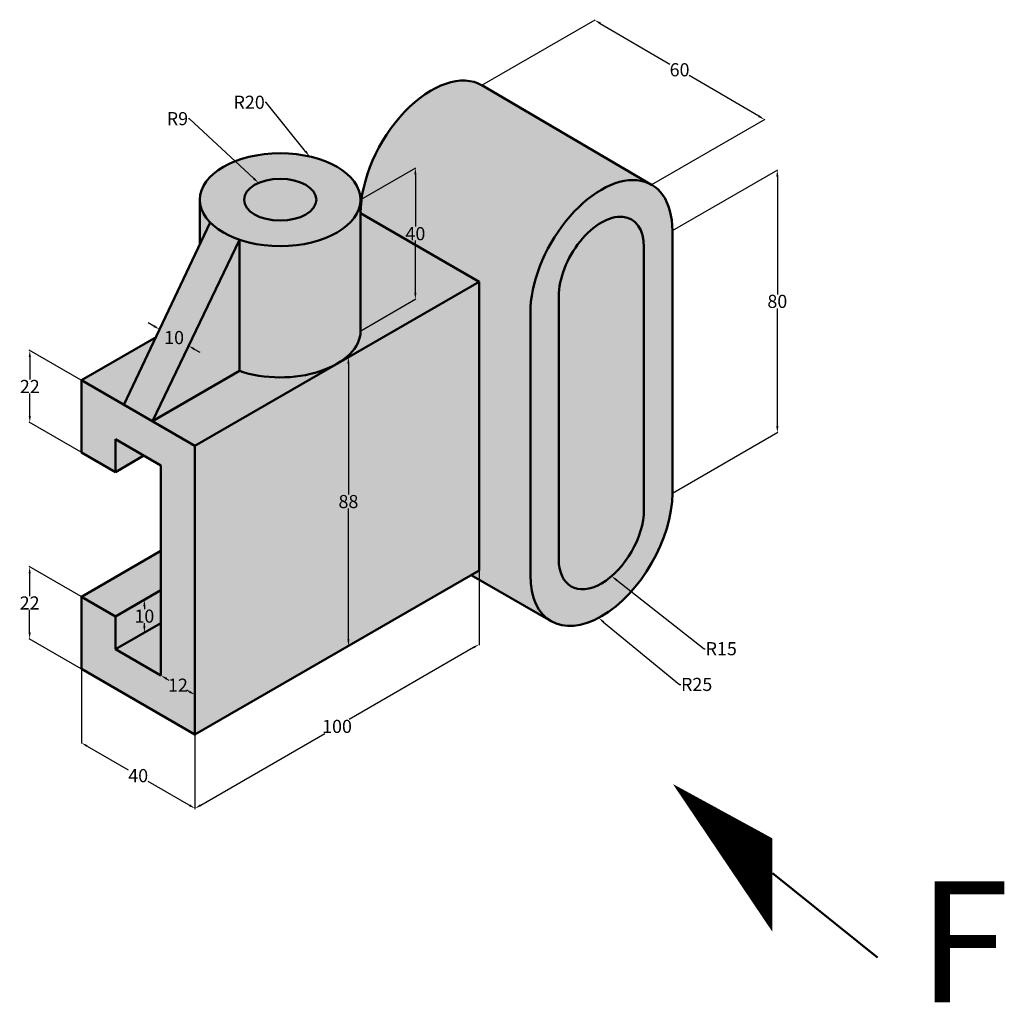
# Model space of a CAD drawing. Units: millimetres. Extents: x -141 to 252, y -566 to 219.
# Tile 2 of 2: x -48 to 252, y -81 to 219. Entities that reach past the tile are written whole.
import ezdxf
from ezdxf import colors
from ezdxf.entities.mleader import LeaderData, LeaderLine
from ezdxf.math import Vec2, Vec3

# ---------------------------------------------------------------- set-up
doc = ezdxf.new("R2010")
doc.units = ezdxf.units.MM
doc.header["$MEASUREMENT"] = 0
for name, color, linetype, lineweight in [('M-DIMS', 2, 'Continuous', 25), ('M-HATC', 141, 'Continuous', 18), ('M-OUTL', 7, 'Continuous', 50), ('M-TEXT', 7, 'Continuous', 25)]:
    doc.layers.add(name, color=color, linetype=linetype, lineweight=lineweight)
doc.styles.get("Standard").update_dxf_attribs({"font": 'arial.ttf'})
doc.dimstyles.get("Standard").update_dxf_attribs({"dimtxt": 4, "dimasz": 2, "dimexe": 0.18, "dimexo": 0.0625, "dimgap": 0.09, "dimtad": 0, "dimtih": 1, "dimtoh": 1, "dimdec": 0, "dimzin": 0, "dimdsep": 46, "dimtxsty": 'Standard', "dimcen": 0.09, "dimadec": 0, "dimazin": 0, "dimtfac": 1, "dimtdec": 0, "dimtofl": 0, "dimtmove": 0, "dimatfit": 3, "dimfxl": 1, "dimtolj": 1, "dimtzin": 0, "dimarcsym": 0})

# ---------------------------------------------------------------- blocks, each defined once
blk = doc.blocks.new('*D1')
at = {"layer": 'Defpoints', "color": 0, "transparency": 16777216}
for p in [(126.9483561768117, 218.4120283637085), (92.53053074867505, 198.5408875878523), (144.304804938695, 168.224989400058)]:
    blk.add_point(p, dxfattribs=at)
at = {"layer": 'M-DIMS', "color": 0, "lineweight": -2, "transparency": 16777216}
for p, q in [((92.5928118403119, 198.5768455928742), (127.1277257207258, 218.5155874181718)), ((128.6742542143024, 217.4014463709016), (149.8764618939226, 204.9867099129304)), ((176.9967323293409, 189.1067121687211), (155.7945246497207, 201.5214486266923)), ((144.3670860303318, 168.2609474050799), (178.9019999107457, 188.1996892303774))]:
    blk.add_line(p, q, dxfattribs=at)
at = {"layer": 'M-DIMS', "color": 0, "transparency": 16777216}
for points in [[(128.8426845464369, 217.6890960438167), (128.505823882168, 217.1137966979865), (126.9483561768117, 218.4120283637085)], [(177.1651626614754, 189.3943618416362), (176.8283019972064, 188.819062495806), (178.7226303668316, 188.0961301759142)]]:
    blk.add_solid(points, dxfattribs=at)
at = {"layer": 'M-DIMS', "color": 0, "transparency": 16777216, "insert": (152.8354932718217, 203.2540792698114), "char_height": 4, "attachment_point": 5}
blk.add_mtext('\\A1;60', dxfattribs=at)
blk = doc.blocks.new('*D2')
at = {"layer": 'Defpoints', "color": 0, "transparency": 16777216}
for p in [(91.69746559874818, 50.66651891708767), (91.69746559874818, 28.15781362692485), (5.094925220304276, 0.6665189170877002)]:
    blk.add_point(p, dxfattribs=at)
at = {"layer": 'M-DIMS', "color": 0, "lineweight": -2, "transparency": 16777216}
for p, q in [((91.69746559874818, 50.59435013343897), (91.69746559874817, 27.94996753001659)), ((89.96541479117931, 27.15781362692486), (52.08943340503227, 5.290105577811644)), ((5.094925220304276, 0.5943501334389967), (5.094925220304275, -22.05003246998336)), ((6.826976027873154, -20.8421863730751), (44.70295741402019, 1.025521676038113))]:
    blk.add_line(p, q, dxfattribs=at)
at = {"layer": 'M-DIMS', "color": 0, "transparency": 16777216}
for points in [[(89.79874812451264, 27.44648876151967), (90.13208145784597, 26.86913849233004), (91.69746559874818, 28.15781362692485)], [(6.660309361206488, -20.55351123848029), (6.99364269453982, -21.13086150766991), (5.094925220304276, -21.8421863730751)]]:
    blk.add_solid(points, dxfattribs=at)
at = {"layer": 'M-DIMS', "color": 0, "transparency": 16777216, "insert": (48.39619540952622, 3.157813626924873), "char_height": 4, "attachment_point": 5}
blk.add_mtext('\\A1;100', dxfattribs=at)
blk = doc.blocks.new('*D3')
at = {"layer": 'Defpoints', "color": 0, "transparency": 16777216}
for p in [(182.6471912993318, 172.6843069570805), (150.6461291409112, 154.2084851055625), (150.6461291409112, 74.20848510556246)]:
    blk.add_point(p, dxfattribs=at)
at = {"layer": 'M-DIMS', "color": 0, "lineweight": -2, "transparency": 16777216}
for p, q in [((150.7086291409112, 154.2445694973868), (182.8271912993318, 172.7882300055346)), ((182.6471912993318, 170.6843069570805), (182.6471912993318, 134.8165989079673)), ((182.6471912993318, 94.68430695708054), (182.6471912993318, 130.5520150061938)), ((150.7086291409112, 74.2445694973868), (182.8271912993318, 92.78823000553464))]:
    blk.add_line(p, q, dxfattribs=at)
at = {"layer": 'M-DIMS', "color": 0, "transparency": 16777216}
for points in [[(182.3138579659985, 170.6843069570805), (182.9805246326652, 170.6843069570805), (182.6471912993318, 172.6843069570805)], [(182.3138579659985, 94.68430695708054), (182.9805246326652, 94.68430695708054), (182.6471912993318, 92.68430695708054)]]:
    blk.add_solid(points, dxfattribs=at)
at = {"layer": 'M-DIMS', "color": 0, "transparency": 16777216, "insert": (182.6471912993318, 132.6843069570805), "char_height": 4, "attachment_point": 5}
blk.add_mtext('\\A1;80', dxfattribs=at)
blk = doc.blocks.new('*D4')
at = {"layer": 'Defpoints', "color": 0, "transparency": 16777216}
for p in [(51.87793235716096, 115.6767006810521), (5.094925220304277, 88.66651891708773), (5.094925220304277, 0.6665189170877002)]:
    blk.add_point(p, dxfattribs=at)
at = {"layer": 'M-DIMS', "color": 0, "lineweight": -2, "transparency": 16777216}
for p, q in [((5.157425220304277, 88.70260330891207), (52.05793235716096, 115.7806237295062)), ((51.87793235716096, 113.6767006810521), (51.87793235716097, 73.80899263193885)), ((51.87793235716098, 29.67670068105207), (51.87793235716097, 69.54440873016532)), ((5.157425220304277, 0.7026033089120518), (52.05793235716098, 27.7806237295062))]:
    blk.add_line(p, q, dxfattribs=at)
at = {"layer": 'M-DIMS', "color": 0, "transparency": 16777216}
for points in [[(51.54459902382762, 113.6767006810521), (52.21126569049429, 113.6767006810521), (51.87793235716096, 115.6767006810521)], [(51.54459902382765, 29.67670068105207), (52.21126569049431, 29.67670068105207), (51.87793235716098, 27.67670068105207)]]:
    blk.add_solid(points, dxfattribs=at)
at = {"layer": 'M-DIMS', "color": 0, "transparency": 16777216, "insert": (51.87793235716098, 71.67670068105205), "char_height": 4, "attachment_point": 5}
blk.add_mtext('\\A1;88', dxfattribs=at)
blk = doc.blocks.new('*D5')
at = {"layer": 'Defpoints', "color": 0, "transparency": 16777216}
for p in [(-29.54609093107331, 20.66651891708764), (5.094925220304276, 0.6665189170876995), (-29.54609093107332, -1.84218637307522)]:
    blk.add_point(p, dxfattribs=at)
at = {"layer": 'M-DIMS', "color": 0, "lineweight": -2, "transparency": 16777216}
for p, q in [((-29.54609093107331, 20.59435013343894), (-29.54609093107331, -2.050032469983486)), ((5.094925220304276, 0.5943501334389967), (5.094925220304276, -22.0500324699834)), ((-27.81404012350444, -2.842186373075215), (-15.2541913137747, -10.09361846435364)), ((3.362874412735394, -20.84218637307515), (-9.196974396994344, -13.59075428179671))]:
    blk.add_line(p, q, dxfattribs=at)
at = {"layer": 'M-DIMS', "color": 0, "transparency": 16777216}
for points in [[(-27.64737345683777, -2.553511238480403), (-27.9807067901711, -3.130861507670028), (-29.54609093107332, -1.84218637307522)], [(3.52954107940206, -20.55351123848033), (3.196207746068729, -21.13086150766996), (5.094925220304274, -21.84218637307514)]]:
    blk.add_solid(points, dxfattribs=at)
at = {"layer": 'M-DIMS', "color": 0, "transparency": 16777216, "insert": (-12.22558285538452, -11.84218637307518), "char_height": 4, "attachment_point": 5}
blk.add_mtext('\\A1;40', dxfattribs=at)
blk = doc.blocks.new('*D6')
at = {"layer": 'Defpoints', "color": 0, "transparency": 16777216}
for p in [(-29.54609093107332, 42.66651891708765), (-45.32566583215914, 29.7768607339274), (-29.54609093107332, 20.66651891708765)]:
    blk.add_point(p, dxfattribs=at)
at = {"layer": 'M-DIMS', "color": 0, "lineweight": -2, "transparency": 16777216}
for p, q in [((-29.60859093107332, 42.70260330891201), (-45.50566583215915, 51.88078378238155)), ((-45.32566583215915, 49.77686073392741), (-45.32566583215914, 42.87504627280871)), ((-45.32566583215914, 31.7768607339274), (-45.32566583215914, 38.6786751950461)), ((-29.60859093107332, 20.702603308912), (-45.50566583215914, 29.88078378238153))]:
    blk.add_line(p, q, dxfattribs=at)
at = {"layer": 'M-DIMS', "color": 0, "transparency": 16777216}
for points in [[(-45.65899916549248, 49.77686073392741), (-44.99233249882581, 49.77686073392741), (-45.32566583215915, 51.77686073392742)], [(-45.65899916549247, 31.7768607339274), (-44.99233249882581, 31.7768607339274), (-45.32566583215914, 29.7768607339274)]]:
    blk.add_solid(points, dxfattribs=at)
at = {"layer": 'M-DIMS', "color": 0, "transparency": 16777216, "insert": (-45.32566583215912, 40.7768607339274), "char_height": 4, "attachment_point": 5}
blk.add_mtext('\\A1;22', dxfattribs=at)
blk = doc.blocks.new('*D7')
at = {"layer": 'Defpoints', "color": 0, "transparency": 16777216}
for p in [(-45.27084352143182, 117.7452090580715), (-29.54609093107329, 108.6665189170877), (-29.54609093107329, 86.66651891708771)]:
    blk.add_point(p, dxfattribs=at)
at = {"layer": 'M-DIMS', "color": 0, "lineweight": -2, "transparency": 16777216}
for p, q in [((-29.60859093107329, 108.7026033089121), (-45.45084352143182, 117.8491321065256)), ((-45.27084352143182, 115.7452090580715), (-45.27084352143181, 108.8433945969528)), ((-45.27084352143181, 97.7452090580715), (-45.27084352143181, 104.6470235191902)), ((-29.60859093107329, 86.70260330891207), (-45.45084352143181, 95.8491321065256))]:
    blk.add_line(p, q, dxfattribs=at)
at = {"layer": 'M-DIMS', "color": 0, "transparency": 16777216}
for points in [[(-45.60417685476515, 115.7452090580715), (-44.93751018809848, 115.7452090580715), (-45.27084352143182, 117.7452090580715)], [(-45.60417685476514, 97.7452090580715), (-44.93751018809848, 97.7452090580715), (-45.27084352143181, 95.74520905807147)]]:
    blk.add_solid(points, dxfattribs=at)
at = {"layer": 'M-DIMS', "color": 0, "transparency": 16777216, "insert": (-45.27084352143178, 106.7452090580714), "char_height": 4, "attachment_point": 5}
blk.add_mtext('\\A1;22', dxfattribs=at)
blk = doc.blocks.new('*D8')
at = {"layer": 'Defpoints', "color": 0, "transparency": 16777216}
for p in [(-5.297379625109019, 18.66651891708764), (5.094925220304275, 12.78049008426763), (5.094925220304275, 12.78049008426763)]:
    blk.add_point(p, dxfattribs=at)
at = {"layer": 'M-DIMS', "color": 0, "lineweight": -2, "transparency": 16777216}
for p, q in [((-5.297379625109018, 18.73834743854851), (-5.297379625109018, 18.87338505889494)), ((-3.557123840112778, 17.68086694869965), (-2.847434569387365, 17.27891073475386)), ((3.354669435308036, 13.76614205265562), (2.644980164582621, 14.16809826660141)), ((5.094925220304275, 12.85231860572849), (5.094925220304275, 12.98735622607492))]:
    blk.add_line(p, q, dxfattribs=at)
at = {"layer": 'M-DIMS', "color": 0, "transparency": 16777216}
for points in [[(-3.392848512048112, 17.97090957953235), (-3.721399168177443, 17.39082431786694), (-5.297379625109018, 18.66651891708764)], [(3.518944763372702, 14.05618468348833), (3.190394107243371, 13.47609942182291), (5.094925220304275, 12.78049008426763)]]:
    blk.add_solid(points, dxfattribs=at)
at = {"layer": 'M-DIMS', "color": 0, "transparency": 16777216, "insert": (-0.1012272024023701, 15.72350450067763), "char_height": 4, "attachment_point": 5}
blk.add_mtext('\\A1;12', dxfattribs=at)
blk = doc.blocks.new('*D9')
at = {"layer": 'Defpoints', "color": 0, "transparency": 16777216}
for p in [(-19.15378608566005, 36.66651891708766), (-10.34520281765164, 31.75215683805154), (-19.15378608566005, 26.66651891708766)]:
    blk.add_point(p, dxfattribs=at)
at = {"layer": 'M-DIMS', "color": 0, "lineweight": -2, "transparency": 16777216}
for p, q in [((-19.09128608566005, 36.70260330891201), (-10.16520281765164, 41.85607988650567)), ((-10.34520281765164, 39.75215683805155), (-10.34520281765164, 38.88444878893831)), ((-10.34520281765164, 33.75215683805154), (-10.34520281765164, 34.61986488716477)), ((-19.09128608566005, 26.70260330891201), (-10.16520281765164, 31.85607988650567))]:
    blk.add_line(p, q, dxfattribs=at)
at = {"layer": 'M-DIMS', "color": 0, "transparency": 16777216}
for points in [[(-10.67853615098497, 39.75215683805155), (-10.01186948431831, 39.75215683805155), (-10.34520281765164, 41.75215683805155)], [(-10.67853615098497, 33.75215683805154), (-10.0118694843183, 33.75215683805154), (-10.34520281765164, 31.75215683805154)]]:
    blk.add_solid(points, dxfattribs=at)
at = {"layer": 'M-DIMS', "color": 0, "transparency": 16777216, "insert": (-10.34520281765163, 36.75215683805153), "char_height": 4, "attachment_point": 5}
blk.add_mtext('\\A1;10', dxfattribs=at)
blk = doc.blocks.new('*D10')
at = {"layer": 'Defpoints', "color": 0, "transparency": 16777216}
for p in [(-6.78467555020569, 121.8078282143685), (3.111764237019578, 119.1474340940985), (2.001825524735131, 116.8026886453206)]:
    blk.add_point(p, dxfattribs=at)
at = {"layer": 'M-DIMS', "color": 0, "lineweight": -2, "transparency": 16777216}
for p, q in [((-7.412560714558523, 125.1425070820132), (-9.150384591195795, 126.1324405008801)), ((-6.757857767013106, 121.8644807794076), (-5.597501622326589, 124.3157330504591)), ((2.028643307927715, 116.8593412103597), (3.188999452614233, 119.3105934814112)), ((4.849588113656857, 118.1575006752317), (6.587411990294128, 117.1675672563649))]:
    blk.add_line(p, q, dxfattribs=at)
at = {"layer": 'M-DIMS', "color": 0, "transparency": 16777216}
for points in [[(-7.247571811414054, 125.4321443947861), (-7.577549617702999, 124.8528697692404), (-5.674736837921251, 124.1525736631464)], [(5.014577016801325, 118.4471379880046), (4.684599210512381, 117.8678633624588), (3.111764237019578, 119.1474340940985)]]:
    blk.add_solid(points, dxfattribs=at)
at = {"layer": 'M-DIMS', "color": 0, "transparency": 16777216, "insert": (-1.281486300450843, 121.6500038786225), "char_height": 4, "attachment_point": 5}
blk.add_mtext('\\A1;10', dxfattribs=at)
blk = doc.blocks.new('*D11')
at = {"layer": 'Defpoints', "color": 0, "transparency": 16777216}
for p in [(55.57058476166926, 163.6665189170877), (72.29189906780866, 133.3205742329416), (55.57058476166926, 123.6665189170877)]:
    blk.add_point(p, dxfattribs=at)
at = {"layer": 'M-DIMS', "color": 0, "lineweight": -2, "transparency": 16777216}
for p, q in [((55.63308476166927, 163.7026033089121), (72.47189906780864, 173.4244972813958)), ((72.29189906780864, 171.3205742329416), (72.29189906780866, 155.4528661838284)), ((72.29189906780866, 135.3205742329416), (72.29189906780866, 151.1882822820549)), ((55.63308476166927, 123.702603308912), (72.47189906780865, 133.4244972813958))]:
    blk.add_line(p, q, dxfattribs=at)
at = {"layer": 'M-DIMS', "color": 0, "transparency": 16777216}
for points in [[(71.95856573447531, 171.3205742329416), (72.62523240114197, 171.3205742329416), (72.29189906780864, 173.3205742329416)], [(71.95856573447533, 135.3205742329416), (72.62523240114199, 135.3205742329416), (72.29189906780866, 133.3205742329416)]]:
    blk.add_solid(points, dxfattribs=at)
at = {"layer": 'M-DIMS', "color": 0, "transparency": 16777216, "insert": (72.29189906780869, 153.3205742329416), "char_height": 4, "attachment_point": 5}
blk.add_mtext('\\A1;40', dxfattribs=at)

msp = doc.modelspace()

# ---------------------------------------------------------------- hatches: boundary and pattern name
at = {"layer": 'M-HATC'}
h = msp.add_hatch(color=256, dxfattribs=at)
h.dxf.hatch_style = 1
edge = h.paths.add_edge_path()
edge.add_ellipse((128.9954940463001, 141.7084851055624), major_axis=(-15.30931089239485, -26.51650429449557), ratio=0.577350269189626, start_angle=180.0000000000107, end_angle=329.99999999999994, ccw=False)
edge.add_line((144.3048049386902, 168.2249894000608), (92.53053074868171, 198.5408875878484))
edge.add_ellipse((77.22121985628019, 172.0243832933567), major_axis=(-15.30931089239485, -26.51650429449557), ratio=0.577350269189626, start_angle=179.9999999999858, end_angle=329.9999999999999)
edge.add_line((55.57058476166924, 159.5243832933566), (91.69746559874818, 138.6665189170877))
edge.add_line((91.69746559874818, 138.6665189170877), (91.69746559874818, 50.66651891708764))
edge.add_line((91.69746559874818, 50.66651891708764), (89.2904812646824, 49.27684586387957))
edge.add_line((89.2904812646824, 49.27684586387957), (113.6861831539054, 35.1919808110668))
edge.add_ellipse((128.9954940463001, 61.70848510556243), major_axis=(-15.30931089239485, -26.51650429449555), ratio=0.5773502691896262, start_angle=330, end_angle=359.99999999999994, ccw=False)
edge.add_line((107.3448589516893, 49.20848510555993), (107.3448589516893, 129.2084851055631))
edge = h.paths.add_edge_path()
edge.add_ellipse((128.9954940463001, 141.7084851055624), major_axis=(-15.30931089239485, -26.51650429449557), ratio=0.577350269189626, start_angle=149.9999999999998, end_angle=179.9999999999879)
edge.add_ellipse((128.9954940463001, 141.7084851055624), major_axis=(-15.30931089239485, -26.51650429449557), ratio=0.577350269189626, start_angle=179.9999999999879, end_angle=329.9999999999999)
edge.add_line((107.3448589516893, 129.2084851055618), (107.3448589516893, 49.20848510555834))
edge.add_ellipse((128.9954940463001, 61.70848510556243), major_axis=(-15.30931089239485, -26.51650429449555), ratio=0.5773502691896262, start_angle=330, end_angle=360)
edge.add_ellipse((128.9954940463001, 61.70848510556243), major_axis=(-15.30931089239485, -26.51650429449555), ratio=0.5773502691896262, start_angle=360, end_angle=417.4938697725578)
edge.add_ellipse((128.9954940463001, 61.70848510556243), major_axis=(-15.30931089239485, -26.51650429449555), ratio=0.5773502691896262, start_angle=417.4938697725578, end_angle=509.9999999999999)
edge.add_line((150.6461291409111, 74.20848510556235), (150.6461291409113, 154.2084851055615))
edge = h.paths.add_edge_path(flags=16)
edge.add_ellipse((128.9954940463001, 141.7084851055624), major_axis=(-9.185586535436894, -15.90990257669734), ratio=0.5773502691896258, start_angle=149.9999999999998, end_angle=329.9999999999999, ccw=False)
edge.add_line((141.9858751030667, 149.2084851055617), (141.9858751030668, 69.20848510556081))
edge.add_ellipse((128.9954940463001, 61.70848510556243), major_axis=(-9.18558653543691, -15.90990257669732), ratio=0.5773502691896263, start_angle=329.99999999999994, end_angle=509.9999999999999, ccw=False)
edge.add_line((116.0051129895337, 54.20848510556237), (116.0051129895336, 134.2084851055621))
h.paths.add_polyline_path([(91.69746559874807, 138.6665189170876), (5.094925220304276, 88.66651891708771), (5.094925220304276, 0.6665189170876431), (91.69746559874818, 50.66651891708762)])
edge = h.paths.add_edge_path()
edge.add_line((91.6974655987483, 138.6665189170877), (55.57058476166924, 159.5243832933566))
edge.add_line((55.57058476166924, 159.5243832933566), (55.57058476166924, 123.6665189170879))
edge.add_ellipse((31.07568733383744, 123.6665189170876), major_axis=(-24.49489742783178, 0), ratio=0.577350269189626, start_angle=150, end_angle=180, ccw=False)
edge.add_line((48.39619540952663, 113.6665189170878), (91.6974655987483, 138.6665189170877))
edge = h.paths.add_edge_path()
edge.add_ellipse((31.07568733383744, 123.6665189170876), major_axis=(-24.49489742783178, 0), ratio=0.577350269189626, start_angle=150, end_angle=180)
edge.add_line((55.57058476166924, 123.6665189170874), (55.57058476166924, 159.5243832933566))
edge.add_line((55.57058476166924, 159.5243832933566), (55.57058476166924, 163.6665189170878))
edge.add_ellipse((31.07568733383744, 163.6665189170876), major_axis=(-24.49489742783178, 0), ratio=0.577350269189626, start_angle=44.399848228089525, end_angle=180, ccw=False)
edge.add_line((18.63530452151121, 151.4840605515691), (18.63530452151121, 111.4840605515691))
edge.add_ellipse((31.07568733383744, 123.6665189170876), major_axis=(-24.49489742783178, 0), ratio=0.577350269189626, start_angle=44.39984822808952, end_angle=150)
h.paths.add_polyline_path([(91.69746559874795, 138.6665189170876), (48.39619540952663, 113.6665189170878), (5.094925220304276, 88.66651891708777), (5.094925220304276, 0.6665189170875863), (91.69746559874818, 50.66651891708762)])
edge = h.paths.add_edge_path(flags=17)
edge.add_ellipse((31.07568733383744, 163.6665189170876), major_axis=(-24.49489742783178, 0), ratio=0.577350269189626, start_angle=44.39984822808948, end_angle=180)
edge.add_ellipse((31.07568733383744, 163.6665189170876), major_axis=(-24.49489742783178, 0), ratio=0.577350269189626, start_angle=180, end_angle=319.5010502042298)
edge.add_ellipse((31.07568733383744, 163.6665189170876), major_axis=(-24.49489742783178, 0), ratio=0.577350269189626, start_angle=319.5010502042298, end_angle=360)
edge.add_ellipse((31.07568733383744, 163.6665189170876), major_axis=(-24.49489742783178, 0), ratio=0.577350269189626, start_angle=0, end_angle=18.03915513234074)
edge.add_ellipse((31.07568733383744, 163.6665189170876), major_axis=(-24.49489742783178, 0), ratio=0.577350269189626, start_angle=18.03915513234074, end_angle=44.39984822808948)
edge = h.paths.add_edge_path(flags=0)
edge.add_ellipse((31.07568733383744, 163.6665189170876), major_axis=(-11.0227038425243, 0), ratio=0.5773502691896253, start_angle=0, end_angle=360)
edge = h.paths.add_edge_path(flags=16)
edge.add_ellipse((31.07568733383744, 163.6665189170876), major_axis=(-11.0227038425243, 0), ratio=0.5773502691896253, start_angle=0, end_angle=360)
h.paths.add_polyline_path([(5.094925220304276, 88.66651891708776), (-29.54609093107331, 108.6665189170877), (-29.54609093107331, 86.66651891708761), (-19.15378608566004, 80.66651891708771), (-19.15378608566004, 90.66651891708767), (-5.297379625108987, 82.66651891708766), (-5.297379625108987, 18.66651891708764), (-19.15378608566004, 26.66651891708764), (-19.15378608566004, 36.66651891708767), (-29.54609093107331, 42.66651891708764), (-29.54609093107331, 20.66651891708762), (5.094925220304276, 0.6665189170877284)])
h.paths.add_polyline_path([(-5.297379625108987, 56.66651891708767), (-29.54609093107331, 42.66651891708764), (-19.15378608566004, 36.66651891708767), (-5.297379625108987, 44.66651891708761)], flags=17)
h.paths.add_polyline_path([(-5.297379625108987, 34.66651891708759), (-5.297379625108874, 44.66651891708752), (-19.15378608566004, 36.66651891708764), (-19.15378608566004, 26.66651891708759)], flags=17)
h.paths.add_polyline_path([(-5.297379625108987, 34.66651891708762), (-19.15378608566004, 26.66651891708759), (-5.297379625108987, 18.66651891708767)], flags=17)
h.paths.add_polyline_path([(-10.49353204781562, 85.66651891708769), (-19.15378608566004, 90.66651891708761), (-19.15378608566004, 80.66651891708771)], flags=17)
edge = h.paths.add_edge_path()
edge.add_ellipse((31.07568733383744, 163.6665189170876), major_axis=(-24.49489742783178, 0), ratio=0.577350269189626, start_angle=18.039155132340795, end_angle=44.399848228089525, ccw=False)
edge.add_line((9.741010934576707, 156.718339708623), (-16.55570987430667, 101.1665189170877))
edge.add_line((-16.55570987430667, 101.1665189170877), (-7.89545583646236, 96.16651891708777))
edge.add_line((-7.89545583646236, 96.16651891708777), (18.63530452151121, 151.4840605515691))
h.paths.add_polyline_path([(-6.784675550205406, 121.8078282143686), (-29.54609093107331, 108.6665189170877), (-16.55570987430667, 101.1665189170876)])
h.paths.add_polyline_path([(18.63530452151121, 111.4840605515692), (18.63530452151121, 151.4840605515689), (-7.895455836462474, 96.16651891708764)], flags=17)
edge = h.paths.add_edge_path()
edge.add_ellipse((31.07568733383744, 123.6665189170876), major_axis=(-24.49489742783178, 0), ratio=0.577350269189626, start_angle=44.399848228089525, end_angle=149.9999999999998, ccw=False)
edge.add_line((18.63530452151121, 111.4840605515691), (-7.895455836462474, 96.16651891708776))
edge.add_line((-7.895455836462474, 96.16651891708776), (5.094925220304276, 88.66651891708779))
edge.add_line((5.094925220304276, 88.66651891708779), (48.39619540952696, 113.6665189170882))
edge = h.paths.add_edge_path(flags=0)
edge.add_ellipse((128.9954940463001, 141.7084851055624), major_axis=(-9.185586535436894, -15.90990257669734), ratio=0.5773502691896258, start_angle=149.9999999999998, end_angle=329.9999999999999)
edge.add_line((116.0051129895337, 134.2084851055628), (116.0051129895337, 54.20848510556178))
edge.add_ellipse((128.9954940463001, 61.70848510556243), major_axis=(-9.18558653543691, -15.90990257669732), ratio=0.5773502691896263, start_angle=329.9999999999999, end_angle=509.9999999999999)
edge.add_line((141.9858751030668, 69.20848510556198), (141.9858751030667, 149.208485105563))
edge = h.paths.add_edge_path()
edge.add_ellipse((31.07568733383744, 163.6665189170876), major_axis=(-24.49489742783178, 0), ratio=0.577350269189626, start_angle=0, end_angle=18.039155132340795, ccw=False)
edge.add_line((6.580789906005634, 163.6665189170877), (6.580789906005634, 150.0423730161707))
edge.add_line((6.580789906005634, 150.0423730161707), (9.741010934576707, 156.7183397086229))
edge = h.paths.add_edge_path()
edge.add_ellipse((31.07568733383744, 163.6665189170876), major_axis=(-24.49489742783178, 0), ratio=0.577350269189626, start_angle=44.39984822808948, end_angle=180)
edge.add_ellipse((31.07568733383744, 163.6665189170876), major_axis=(-24.49489742783178, 0), ratio=0.577350269189626, start_angle=180, end_angle=404.3998482280894)
h = msp.add_hatch(color=256, dxfattribs=at)
h.dxf.hatch_style = 1
edge = h.paths.add_edge_path()
edge.add_ellipse((31.07568733383744, 163.6665189170876), major_axis=(-24.49489742783178, 0), ratio=0.577350269189626, start_angle=44.39984822808948, end_angle=180)
edge.add_ellipse((31.07568733383744, 163.6665189170876), major_axis=(-24.49489742783178, 0), ratio=0.577350269189626, start_angle=180, end_angle=319.5010502042298)
edge.add_ellipse((31.07568733383744, 163.6665189170876), major_axis=(-24.49489742783178, 0), ratio=0.577350269189626, start_angle=319.5010502042298, end_angle=360)
edge.add_ellipse((31.07568733383744, 163.6665189170876), major_axis=(-24.49489742783178, 0), ratio=0.577350269189626, start_angle=0, end_angle=18.03915513234074)
edge.add_ellipse((31.07568733383744, 163.6665189170876), major_axis=(-24.49489742783178, 0), ratio=0.577350269189626, start_angle=18.03915513234074, end_angle=44.39984822808948)
edge = h.paths.add_edge_path(flags=16)
edge.add_ellipse((31.07568733383744, 163.6665189170876), major_axis=(-11.0227038425243, 0), ratio=0.5773502691896253, start_angle=0, end_angle=360)
h.paths.add_polyline_path([(91.69746559874818, 138.6665189170876), (5.094925220304268, 88.66651891708769), (5.094925220304268, 0.6665189170877), (91.69746559874818, 50.66651891708769)])
edge = h.paths.add_edge_path()
edge.add_ellipse((128.9954940463001, 141.7084851055624), major_axis=(-9.185586535436894, -15.90990257669734), ratio=0.5773502691896258, start_angle=149.9999999999998, end_angle=329.9999999999999)
edge.add_line((116.0051129895336, 134.2084851055621), (116.0051129895336, 54.20848510556246))
edge.add_ellipse((128.9954940463001, 61.70848510556243), major_axis=(-9.18558653543691, -15.90990257669732), ratio=0.5773502691896263, start_angle=329.9999999999999, end_angle=509.9999999999999)
edge.add_line((141.9858751030667, 69.20848510556249), (141.9858751030667, 149.2084851055623))

# ---------------------------------------------------------------- linework, layer by layer
at = {"layer": 'M-OUTL'}
for p, q in [((92.53053074867508, 198.5408875878523), (144.304804938695, 168.2249894000579)), ((6.580789906005662, 163.6665189170876), (6.580789906005662, 150.042373016171)), ((55.57058476166924, 163.6665189170876), (55.57058476166924, 123.6665189170876)), ((91.69746559874818, 138.6665189170876), (55.57058476166923, 159.5243832933567)), ((9.741010934576565, 156.718339708623), (-16.5557098743067, 101.1665189170877)), ((150.6461291409111, 74.20848510556243), (150.6461291409111, 154.2084851055624)), ((18.63530452151119, 151.4840605515691), (-7.895455836462303, 96.16651891708769)), ((18.63530452151119, 151.4840605515691), (18.63530452151119, 111.4840605515691)), ((141.9858751030667, 149.2084851055623), (141.9858751030667, 69.20848510556243)), ((91.69746559874818, 138.6665189170876), (5.094925220304276, 88.66651891708769)), ((91.69746559874818, 50.66651891708767), (91.69746559874818, 138.6665189170876)), ((116.0051129895336, 134.2084851055624), (116.0051129895336, 54.20848510556243)), ((107.3448589516892, 129.2084851055624), (107.3448589516892, 49.20848510556243)), ((-29.54609093107328, 108.6665189170877), (-6.784675550205698, 121.8078282143685)), ((-7.895455836462303, 96.16651891708769), (18.63530452151119, 111.4840605515691)), ((5.094925220304276, 88.66651891708769), (-29.54609093107328, 108.6665189170877)), ((-29.54609093107328, 108.6665189170877), (-29.54609093107328, 86.6665189170877)), ((-12.22558285538452, 98.66651891708769), (-16.5557098743067, 101.1665189170877)), ((-19.15378608566001, 80.66651891708771), (-19.15378608566001, 90.66651891708771)), ((-19.15378608566001, 90.66651891708771), (-5.297379625109016, 82.66651891708764)), ((5.094925220304276, 0.666518917087693), (5.094925220304276, 88.66651891708769)), ((-29.54609093107328, 86.6665189170877), (-19.15378608566001, 80.66651891708771)), ((-19.15378608566001, 80.66651891708771), (-10.49353204781566, 85.66651891708769)), ((-5.297379625109016, 82.66651891708764), (-5.297379625109016, 18.66651891708764)), ((-29.54609093107331, 42.66651891708764), (-5.297379625109016, 56.66651891708767)), ((5.094925220304276, 0.6665189170877), (91.69746559874818, 50.66651891708767)), ((113.6861831539053, 35.19198081106689), (89.29048126468241, 49.27684586387958)), ((-19.15378608566004, 36.66651891708764), (-29.54609093107331, 42.66651891708764)), ((-29.54609093107331, 42.66651891708764), (-29.54609093107331, 20.66651891708764)), ((-19.15378608566004, 36.66651891708764), (-5.297379625109017, 44.66651891708763)), ((-19.15378608566004, 26.66651891708764), (-19.15378608566004, 36.66651891708764)), ((-19.15378608566004, 26.66651891708764), (-5.297379625109016, 34.66651891708765)), ((-5.297379625109016, 18.66651891708764), (-19.15378608566004, 26.66651891708764)), ((-29.54609093107331, 20.66651891708764), (5.094925220304276, 0.6665189170877)), ((181.1224976990438, -41.55047939533671), (181.1224976990438, -41.55047939533671)), ((181.1224976990438, -41.55047939533671), (213.1530946294497, -67.22084569033109))]:
    msp.add_line(p, q, dxfattribs=at)
for centre, major_axis, ratio, start_param, end_param in [((77.22121985628019, 172.0243832933567), (-15.30931089239484, -26.51650429449555), 0.577350269189626, 3.134525402505678, 5.497787143782137), ((128.9954940463001, 141.7084851055624), (-15.30931089239484, -26.51650429449555), 0.577350269189626, 2.356194490192341, 5.497787143782137), ((128.9954940463001, 141.7084851055624), (-9.18558653543689, -15.90990257669733), 0.577350269189626, 2.356194490192341, 5.497787143782136), ((31.07568733383744, 123.6665189170876), (-24.49489742783178, 0), 0.577350269189626, 1.038078418539525, 3.141592653589793), ((128.9954940463001, 61.70848510556243), (-15.30931089239484, -26.51650429449554), 0.5773502691896262, 5.497787143782137, 8.63937979737193), ((128.9954940463001, 61.70848510556243), (-9.18558653543691, -15.90990257669732), 0.5773502691896263, 5.497787143782137, 8.63937979737193)]:
    msp.add_ellipse(centre, major_axis=major_axis, ratio=ratio, start_param=start_param, end_param=end_param, dxfattribs=at)
for major_axis, ratio in [((-24.49489742783178, 0), 0.577350269189626), ((-11.0227038425243, 0), 0.5773502691896253)]:
    msp.add_ellipse((31.07568733383744, 163.6665189170876), major_axis=major_axis, ratio=ratio, dxfattribs=at)
at = {"layer": 'M-TEXT'}
msp.add_lwpolyline([(181.1224976990438, -41.08226044179002, 0, 0, 0), (181.1224976990438, -42.01869834888339, 20, 0, 0), (150.7989188012157, -14.39952663958024, 0, 0, 0)], format="xyseb", dxfattribs=at)

# ---------------------------------------------------------------- texts
msp.add_text('F', height=36.86743849454149, dxfattribs=at).set_placement((225.5418825802847, -80.91846499343876))

# ---------------------------------------------------------------- dimensions: what is measured, and where the dimension line sits
at = {"layer": 'M-DIMS'}
for p1, p2, distance, picture, middle in [((144.304804938695, 168.2249894000579), (92.53053074867508, 198.5408875878523), -34.538798738499935, '*D1', (152.8354932718217, 203.2540792698114)), ((55.57058476166924, 163.6665189170876), (55.57058476166924, 123.6665189170876), 16.72131430613942, '*D11', (72.29189906780869, 153.3205742329416)), ((150.6461291409111, 74.20848510556243), (150.6461291409111, 154.2084851055624), -32.001062158420694, '*D3', (182.6471912993318, 132.6843069570805)), ((-6.78467555020569, 121.8078282143685), (2.001825524735124, 116.8026886453206), 2.586760024853613, '*D10', (-1.281486300450843, 121.6500038786225)), ((-29.54609093107328, 86.6665189170877), (-29.54609093107328, 108.6665189170877), 15.724752590358541, '*D7', (-45.27084352143178, 106.7452090580714)), ((5.094925220304276, 0.6665189170877), (5.094925220304276, 88.66651891708769), -46.78300713685669, '*D4', (51.87793235716098, 71.67670068105205)), ((-29.54609093107331, 42.66651891708764), (-29.54609093107331, 20.66651891708764), -15.77957490108583, '*D6', (-45.32566583215912, 40.7768607339274)), ((5.094925220304276, 0.6665189170877), (91.69746559874818, 50.66651891708767), -19.493110587578197, '*D2', (48.39619540952622, 3.157813626924873)), ((-19.15378608566004, 36.66651891708764), (-19.15378608566004, 26.66651891708764), 8.808583268008402, '*D9', (-10.34520281765163, 36.75215683805153)), ((5.094925220304276, 0.6665189170877), (-29.54609093107331, 20.66651891708764), 19.493110587578247, '*D5', (-12.22558285538452, -11.84218637307518)), ((-5.297379625109016, 18.66651891708764), (5.094925220304276, 12.78049008426762), 7.73401070418518e-15, '*D8', (-0.1012272024023701, 15.72350450067763))]:
    dim = msp.add_aligned_dim(p1=p1, p2=p2, distance=distance, dimstyle='Standard', override={"dimclrd": 0, "dimclre": 0, "dimclrt": 0}, dxfattribs=at)
    dim.commit()
    dim.dimension.update_dxf_attribs({"geometry": picture, "text_midpoint": middle})

# ---------------------------------------------------------------- leaders
at = {"layer": 'M-TEXT'}
ml = msp.add_multileader_mtext('Standard', dxfattribs=at)
ml.set_content('R20', color=256)
ml.set_leader_properties()
ml.build(insert=Vec2(0, 0))
ml.multileader.update_dxf_attribs({"dogleg_length": 0.36, "arrow_head_size": 2})
ctx = ml.context
ctx.base_point, ctx.arrow_head_size, ctx.landing_gap_size, ctx.plane_origin = Vec3(16.73221350604647, 193.3245869679707), 2, 0.09, Vec3(40.0591863406845, 176.8232250093431)
ctx.text_align_type = 2
notes = []
notes.append((ctx, [(0, (1, 1, 0), (26.81655184165356, 193.3245869679707), (-1, 0), 0.36, [(0, [(40.05918634068449, 176.8232250093431)], 0, [])])]))
ctx.mtext.insert, ctx.mtext.alignment, ctx.mtext.flow_direction = Vec3(26.36655184165356, 195.3586933799762), 3, 5
ml = msp.add_multileader_mtext('Standard', dxfattribs=at)
ml.set_content('R9', color=256)
ml.set_leader_properties()
ml.build(insert=Vec2(0, 0))
ml.multileader.update_dxf_attribs({"dogleg_length": 0.36, "arrow_head_size": 2})
ctx = ml.context
ctx.base_point, ctx.arrow_head_size, ctx.landing_gap_size, ctx.plane_origin = Vec3(-3.561967891670376, 188.3307253875739), 2, 0.09, Vec3(24.47435902179768, 168.763003474004)
ctx.text_align_type = 2
notes.append((ctx, [(0, (1, 1, 0), (3.436422285682965, 188.3307253875739), (-1, 0), 0.36, [(0, [(24.47435902179768, 168.7630034740041)], 0, [])])]))
ctx.mtext.insert, ctx.mtext.alignment, ctx.mtext.flow_direction = Vec3(2.986422285682965, 190.3648317995793), 3, 5
ml = msp.add_multileader_mtext('Standard', dxfattribs=at)
ml.set_content('R15', color=256)
ml.set_leader_properties()
ml.build(insert=Vec2(0, 0))
ml.multileader.update_dxf_attribs({"dogleg_length": 0.36, "arrow_head_size": 2})
ctx = ml.context
ctx.base_point, ctx.arrow_head_size, ctx.landing_gap_size, ctx.plane_origin = Vec3(160.6895314837537, 26.79862412549596), 2, 0.09, Vec3(132.1073633593482, 48.94186996226705)
notes.append((ctx, [(0, (1, 1, 0), (160.3295314837537, 26.79862412549596), (1, 0), 0.36, [(0, [(132.1073633593482, 48.94186996226706)], 0, [])])]))
ctx.mtext.insert, ctx.mtext.flow_direction = Vec3(160.7795314837537, 28.83273053750142), 5
ml = msp.add_multileader_mtext('Standard', dxfattribs=at)
ml.set_content('R25', color=256)
ml.set_leader_properties()
ml.build(insert=Vec2(0, 0))
ml.multileader.update_dxf_attribs({"dogleg_length": 0.36, "arrow_head_size": 2})
ctx = ml.context
ctx.base_point, ctx.arrow_head_size, ctx.landing_gap_size, ctx.plane_origin = Vec3(153.1936121771658, 15.91913965359561), 2, 0.09, Vec3(128.1318711206115, 36.22976928304169)
notes.append((ctx, [(0, (1, 1, 0), (152.8336121771658, 15.91913965359561), (1, 0), 0.36, [(0, [(128.1318711206115, 36.22976928304171)], 0, [])])]))
ctx.mtext.insert, ctx.mtext.flow_direction = Vec3(153.2836121771658, 17.95324606560106), 5
for ctx, leaders in notes:
    for number, flags, end, landing, length, lines in leaders:
        leader = LeaderData()
        leader.index, (leader.has_last_leader_line, leader.has_dogleg_vector, leader.attachment_direction) = number, flags
        leader.last_leader_point, leader.dogleg_vector, leader.dogleg_length = Vec3(end), Vec3(landing), length
        for number, points, colour, breaks in lines:
            line = LeaderLine()
            line.index, line.vertices, line.color, line.breaks = number, Vec3.list(points), colors.encode_raw_color(colour), breaks
            leader.lines.append(line)
        ctx.leaders.append(leader)

doc.saveas('drawing.dxf')
